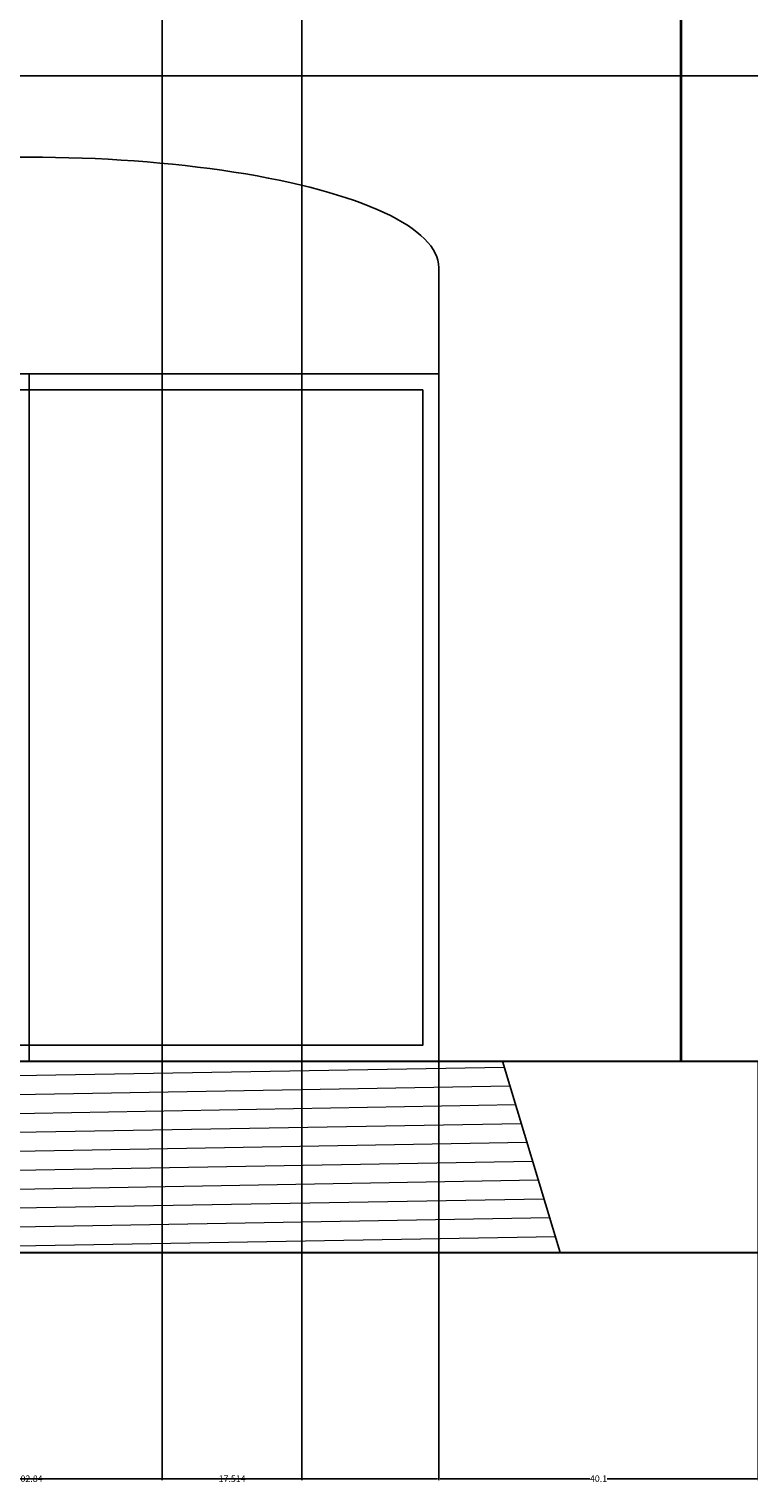
# Model space of a CAD drawing. Units: inches. Extents: x 69 to 650, y -16 to 573.
# Tile 3 of 26: x 174 to 264, y 35 to 218. Entities that reach past the tile are written whole.
import ezdxf

# ---------------------------------------------------------------- set-up
doc = ezdxf.new("R2010")
doc.units = ezdxf.units.IN
doc.header["$MEASUREMENT"] = 0
for name, color, linetype, lineweight in [('A-ANNO-DIMS', 2, 'Continuous', 18), ('A-DOOR', 3, 'Continuous', 25), ('A-FLOR-PATT', 252, 'Continuous', 13), ('A-FLOR-STRS', 7, 'Continuous', 25), ('A-WALL', 7, 'Continuous', 35), ('A-WALL-BASE', 7, 'Continuous', 30)]:
    doc.layers.add(name, color=color, linetype=linetype, lineweight=lineweight)
doc.styles.get("Standard").update_dxf_attribs({"font": 'arial.ttf'})
doc.dimstyles.get("Standard").update_dxf_attribs({"dimtxt": 0.8125, "dimasz": 0.18, "dimexe": 0.18, "dimexo": 0.0625, "dimgap": 0.09, "dimtad": 0, "dimtih": 1, "dimtoh": 1, "dimdec": 4, "dimzin": 0, "dimdsep": 46, "dimlunit": 4, "dimtxsty": 'Standard', "dimcen": 0.09, "dimadec": 0, "dimazin": 0, "dimtfac": 1, "dimtdec": 4, "dimtofl": 0, "dimtmove": 0, "dimatfit": 3, "dimfxl": 1, "dimtolj": 1, "dimtzin": 0, "dimarcsym": 0})

# ---------------------------------------------------------------- blocks, each defined once
blk = doc.blocks.new('*D19')
at = {"layer": 'A-ANNO-DIMS', "color": 0, "lineweight": -2, "transparency": 16777216}
for p, q in [((99.56, 471.72), (99.56, 572.74)), ((99.74, 572.56), (358.57, 572.56)), ((619.38, 572.56), (360.54, 572.56)), ((619.56, 87.99), (619.56, 572.74))]:
    blk.add_line(p, q, dxfattribs=at)
at = {"layer": 'A-ANNO-DIMS', "color": 0, "transparency": 16777216}
for points in [[(99.74, 572.59), (99.74, 572.53), (99.56, 572.56)], [(619.38, 572.59), (619.38, 572.53), (619.56, 572.56)]]:
    blk.add_solid(points, dxfattribs=at)
at = {"layer": 'Defpoints', "color": 0, "transparency": 16777216}
for p in [(619.56, 572.56), (99.56, 471.66), (619.56, 87.93)]:
    blk.add_point(p, dxfattribs=at)
at = {"layer": 'A-ANNO-DIMS', "color": 0, "transparency": 16777216, "insert": (359.56, 572.56), "char_height": 0.812, "attachment_point": 5}
blk.add_mtext('\\A1;520', dxfattribs=at)
blk = doc.blocks.new('*D24')
at = {"layer": 'A-ANNO-DIMS', "color": 0, "lineweight": -2, "transparency": 16777216}
for p, q in [((441.88, 211.65), (70.98, 211.65)), ((71.16, 211.47), (71.16, 207.04)), ((71.16, 201.6), (71.16, 206.03)), ((173.51, 201.42), (70.98, 201.42))]:
    blk.add_line(p, q, dxfattribs=at)
at = {"layer": 'A-ANNO-DIMS', "color": 0, "transparency": 16777216}
for points in [[(71.13, 211.47), (71.19, 211.47), (71.16, 211.65)], [(71.13, 201.6), (71.19, 201.6), (71.16, 201.42)]]:
    blk.add_solid(points, dxfattribs=at)
at = {"layer": 'Defpoints', "color": 0, "transparency": 16777216}
for p in [(71.16, 211.65), (441.94, 211.65), (173.58, 201.42)]:
    blk.add_point(p, dxfattribs=at)
at = {"layer": 'A-ANNO-DIMS', "color": 0, "transparency": 16777216, "insert": (71.16, 206.54), "char_height": 0.812, "attachment_point": 5}
blk.add_mtext('\\A1;10.229', dxfattribs=at)
blk = doc.blocks.new('*D25')
at = {"layer": 'A-ANNO-DIMS', "color": 0, "lineweight": -2, "transparency": 16777216}
for p, q in [((99.49, 243.93), (70.98, 243.93)), ((71.16, 243.75), (71.16, 228.3)), ((71.16, 211.83), (71.16, 227.29)), ((441.88, 211.65), (70.98, 211.65))]:
    blk.add_line(p, q, dxfattribs=at)
at = {"layer": 'A-ANNO-DIMS', "color": 0, "transparency": 16777216}
for points in [[(71.13, 243.75), (71.19, 243.75), (71.16, 243.93)], [(71.13, 211.83), (71.19, 211.83), (71.16, 211.65)]]:
    blk.add_solid(points, dxfattribs=at)
at = {"layer": 'Defpoints', "color": 0, "transparency": 16777216}
for p in [(71.16, 243.93), (99.56, 243.93), (441.94, 211.65)]:
    blk.add_point(p, dxfattribs=at)
at = {"layer": 'A-ANNO-DIMS', "color": 0, "transparency": 16777216, "insert": (71.16, 227.79), "char_height": 0.812, "attachment_point": 5}
blk.add_mtext('\\A1;32.28', dxfattribs=at)
blk = doc.blocks.new('*D27')
at = {"layer": 'A-ANNO-DIMS', "color": 0, "lineweight": -2, "transparency": 16777216}
for p, q in [((122.16, 87.87), (122.16, 35.35)), ((225, 87.87), (225, 35.35)), ((122.34, 35.53), (171.84, 35.53)), ((224.82, 35.53), (175.31, 35.53))]:
    blk.add_line(p, q, dxfattribs=at)
at = {"layer": 'A-ANNO-DIMS', "color": 0, "transparency": 16777216}
for points in [[(122.34, 35.56), (122.34, 35.5), (122.16, 35.53)], [(224.82, 35.56), (224.82, 35.5), (225, 35.53)]]:
    blk.add_solid(points, dxfattribs=at)
at = {"layer": 'Defpoints', "color": 0, "transparency": 16777216}
for p in [(122.16, 87.93), (225, 87.93), (225, 35.53)]:
    blk.add_point(p, dxfattribs=at)
at = {"layer": 'A-ANNO-DIMS', "color": 0, "transparency": 16777216, "insert": (173.58, 35.53), "char_height": 0.812, "attachment_point": 5}
blk.add_mtext('\\A1;102.84', dxfattribs=at)
blk = doc.blocks.new('*D28')
at = {"layer": 'A-ANNO-DIMS', "color": 0, "lineweight": -2, "transparency": 16777216}
for p, q in [((225, 87.87), (225, 35.35)), ((265.1, 87.92), (265.1, 35.35)), ((225.18, 35.53), (243.96, 35.53)), ((264.92, 35.53), (246.13, 35.53))]:
    blk.add_line(p, q, dxfattribs=at)
at = {"layer": 'A-ANNO-DIMS', "color": 0, "transparency": 16777216}
for points in [[(225.18, 35.56), (225.18, 35.5), (225, 35.53)], [(264.92, 35.56), (264.92, 35.5), (265.1, 35.53)]]:
    blk.add_solid(points, dxfattribs=at)
at = {"layer": 'Defpoints', "color": 0, "transparency": 16777216}
for p in [(225, 87.93), (265.1, 87.99), (265.1, 35.53)]:
    blk.add_point(p, dxfattribs=at)
at = {"layer": 'A-ANNO-DIMS', "color": 0, "transparency": 16777216, "insert": (245.05, 35.53), "char_height": 0.812, "attachment_point": 5}
blk.add_mtext('\\A1;40.1', dxfattribs=at)
blk = doc.blocks.new('*D35')
at = {"layer": 'A-ANNO-DIMS', "color": 0, "lineweight": -2, "transparency": 16777216}
for p, q in [((99.56, 243.87), (99.56, 35.35)), ((190.3, 243.87), (190.3, 35.35)), ((99.74, 35.53), (143.47, 35.53)), ((190.12, 35.53), (146.39, 35.53))]:
    blk.add_line(p, q, dxfattribs=at)
at = {"layer": 'A-ANNO-DIMS', "color": 0, "transparency": 16777216}
for points in [[(99.74, 35.56), (99.74, 35.5), (99.56, 35.53)], [(190.12, 35.56), (190.12, 35.5), (190.3, 35.53)]]:
    blk.add_solid(points, dxfattribs=at)
at = {"layer": 'Defpoints', "color": 0, "transparency": 16777216}
for p in [(99.56, 243.93), (190.3, 243.93), (190.3, 35.53)]:
    blk.add_point(p, dxfattribs=at)
at = {"layer": 'A-ANNO-DIMS', "color": 0, "transparency": 16777216, "insert": (144.93, 35.53), "char_height": 0.812, "attachment_point": 5}
blk.add_mtext('\\A1;90.74', dxfattribs=at)
blk = doc.blocks.new('*D36')
at = {"layer": 'A-ANNO-DIMS', "color": 0, "lineweight": -2, "transparency": 16777216}
for p, q in [((207.81, 372.93), (207.81, 35.35)), ((190.3, 243.87), (190.3, 35.35)), ((190.48, 35.53), (197.32, 35.53)), ((207.63, 35.53), (200.79, 35.53))]:
    blk.add_line(p, q, dxfattribs=at)
at = {"layer": 'A-ANNO-DIMS', "color": 0, "transparency": 16777216}
for points in [[(190.48, 35.56), (190.48, 35.5), (190.3, 35.53)], [(207.63, 35.56), (207.63, 35.5), (207.81, 35.53)]]:
    blk.add_solid(points, dxfattribs=at)
at = {"layer": 'Defpoints', "color": 0, "transparency": 16777216}
for p in [(207.81, 372.99), (190.3, 243.93), (207.81, 35.53)]:
    blk.add_point(p, dxfattribs=at)
at = {"layer": 'A-ANNO-DIMS', "color": 0, "transparency": 16777216, "insert": (199.06, 35.53), "char_height": 0.812, "attachment_point": 5}
blk.add_mtext('\\A1;17.514', dxfattribs=at)

msp = doc.modelspace()

# ---------------------------------------------------------------- hatches: boundary and pattern name
at = {"layer": 'A-FLOR-PATT'}
h = msp.add_hatch(dxfattribs=at)
h.set_pattern_fill('ANSI31', color=256, scale=19, angle=136)
h.paths.add_polyline_path([(232.9803, 87.93), (117.2878, 87.93), (99.556, 63.93), (240.241, 63.93)])

# ---------------------------------------------------------------- linework, layer by layer
at = {"layer": 'A-DOOR'}
for p, q in [((224.9972, 174.2116), (224.9972, 187.5532)), ((173.5769, 174.2116), (173.5769, 87.93))]:
    msp.add_line(p, q, dxfattribs=at)
for points in [[(122.1565, 174.2116), (224.9972, 174.2116), (224.9972, 87.93), (122.1565, 87.93)], [(124.1565, 172.2116), (222.9972, 172.2116), (222.9972, 89.93), (124.1565, 89.93)]]:
    msp.add_lwpolyline(points, close=True, dxfattribs=at)
msp.add_ellipse((173.5769, 187.5726), major_axis=(-51.4203, 0.0194), ratio=0.26935388, start_param=3.14159265, end_param=6.28338858, dxfattribs=at)
at = {"layer": 'A-FLOR-STRS'}
msp.add_lwpolyline([(232.9803, 87.93), (240.241, 63.93)], dxfattribs=at)
at = {"layer": 'A-WALL'}
msp.add_line((255.3778, 243.93), (255.3778, 87.93), dxfattribs=at)
at = {"layer": 'A-WALL-BASE'}
for p, q in [((99.556, 87.93), (463.7847, 87.93)), ((99.556, 63.93), (463.7847, 63.93))]:
    msp.add_line(p, q, dxfattribs=at)

# ---------------------------------------------------------------- dimensions: what is measured, and where the dimension line sits
at = {"layer": 'A-ANNO-DIMS'}
for base, p1, p2, override, picture, middle in [((619.555, 572.5573), (99.556, 471.6595), (619.555, 87.93), {"dimdec": 0, "dimlfac": 1, "dimrnd": 0, "dimzin": 0, "dimdsep": 46, "dimlunit": 2}, '*D19', (359.5555, 572.5573)), ((207.8126, 35.53), (190.299, 243.93), (207.8126, 372.9907), {"dimdec": 3, "dimlfac": 1, "dimrnd": 0, "dimzin": 0, "dimdsep": 46, "dimlunit": 2}, '*D36', (199.0558, 35.53)), ((190.299, 35.53), (99.556, 243.93), (190.299, 243.93), {"dimdec": 2, "dimlfac": 1, "dimrnd": 0, "dimzin": 0, "dimdsep": 46, "dimlunit": 2}, '*D35', (144.9275, 35.53)), ((224.9972, 35.53), (122.1565, 87.93), (224.9972, 87.93), {"dimdec": 2, "dimlfac": 1, "dimrnd": 0, "dimzin": 0, "dimdsep": 46, "dimlunit": 2}, '*D27', (173.5769, 35.53)), ((265.0952, 35.53), (224.9972, 87.93), (265.0952, 87.985), {"dimdec": 1, "dimlfac": 1, "dimrnd": 0, "dimzin": 0, "dimdsep": 46, "dimlunit": 2}, '*D28', (245.0462, 35.53))]:
    dim = msp.add_linear_dim(base=base, p1=p1, p2=p2, dimstyle='Standard', override=override, dxfattribs=at)
    dim.commit()
    dim.dimension.update_dxf_attribs({"geometry": picture, "text_midpoint": middle})
for base, p1, p2, override, picture, middle in [((71.156, 243.93), (441.9398, 211.6519), (99.556, 243.93), {"dimdec": 2, "dimlfac": 1, "dimrnd": 0, "dimzin": 0, "dimdsep": 46, "dimlunit": 2}, '*D25', (71.156, 227.7909)), ((71.156, 211.6519), (173.5769, 201.4229), (441.9398, 211.6519), {"dimdec": 3, "dimlfac": 1, "dimrnd": 0, "dimzin": 0, "dimdsep": 46, "dimlunit": 2}, '*D24', (71.156, 206.5374))]:
    dim = msp.add_linear_dim(base=base, p1=p1, p2=p2, angle=90, dimstyle='Standard', override=override, dxfattribs=at)
    dim.commit()
    dim.dimension.update_dxf_attribs({"geometry": picture, "text_midpoint": middle})

doc.saveas('drawing.dxf')
